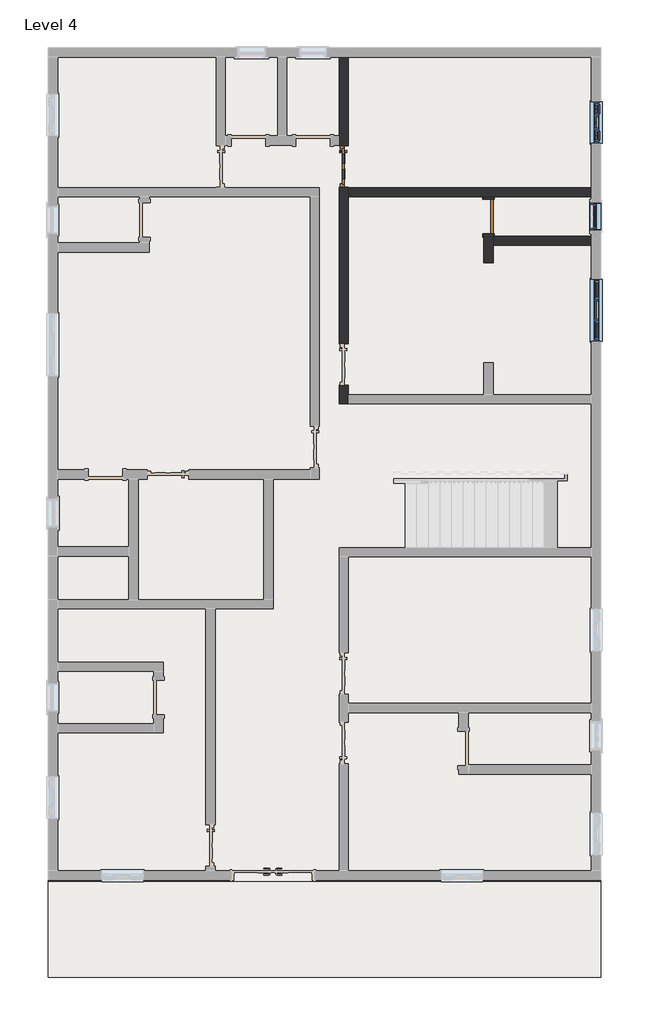
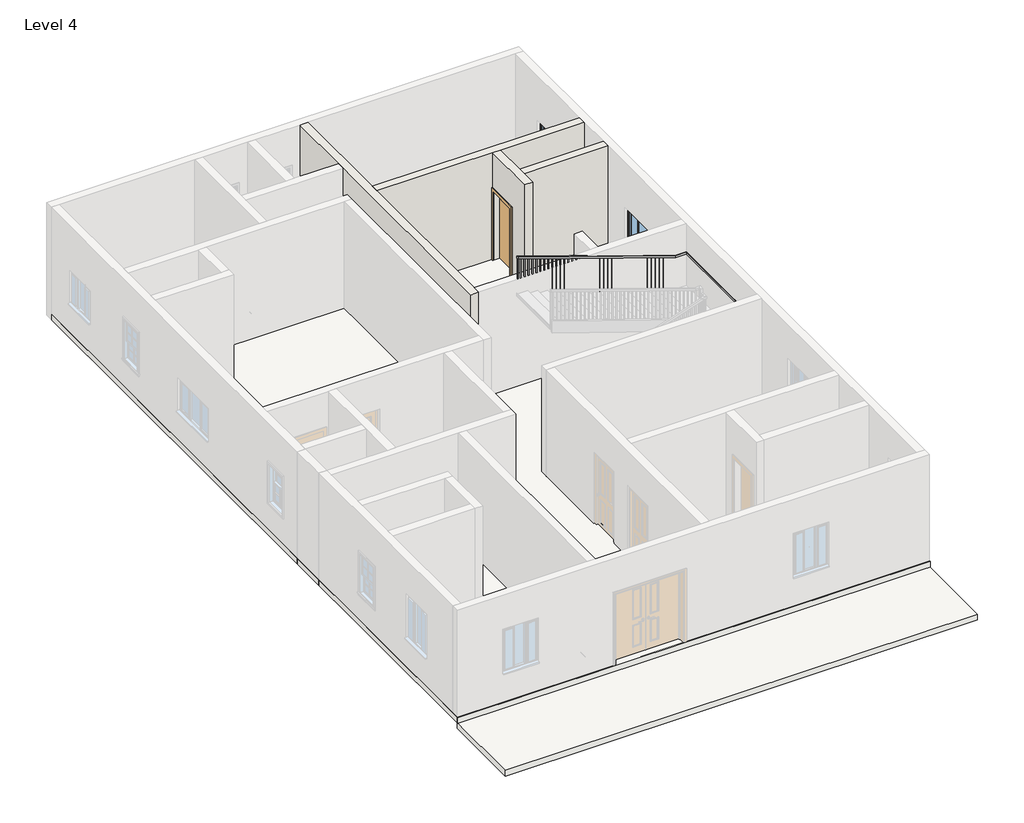
# One storey, part 2 of 3: 4 roofs, 4 walls, 3 windows, 2 doors, 1 railing, 1 slab.
"""IFC4 building model written with IfcOpenShell, lengths in millimetres."""

from ifc_helpers import new_model, si_unit, frame, origin, place, context, project, spatial, polyline, outline, extrude, faceted_brep, transform, mapped, element, save
from components import door_51b0c682, door_fadea3f2, window_679d2811, windows_tpl_plain_1360x910mm_84993ef1, windows_tpl_w_glazing_cross_bars_910x910mm_4aa0f884

model = new_model("IFC4")

# Units and contexts
model_context = context("Model", 3, world=origin())
ifc_project = project(units=[si_unit("LENGTHUNIT", "METRE", prefix="MILLI")], contexts=[model_context])

# Site, building, storey
site = spatial("IfcSite", under=ifc_project)
building = spatial("IfcBuilding", under=site)
storey = spatial("IfcBuildingStorey", under=building, Name="Level 4", Elevation=9144.0)

# Doors
placement = place(None, origin())
door_shape = door_51b0c682(model_context)
element("IfcDoor", 1, ObjectType="Doors_ExtSgl_2 : 2'x7\"", at=placement, inside=storey, context=model_context, shape_type="MappedRepresentation", body=[
    mapped(door_shape, transform((348.5548051, 6357.8803322, 9144.0), x_axis=(0.0, -1.0, 0.0), y_axis=(1.0, 0.0, 0.0), z_axis=(0.0, 0.0, 1.0))),
])
door_2_shape = door_fadea3f2(model_context)
element("IfcDoor", 2, ObjectType="Single-Flush : 30\" x 80\"", at=placement, inside=storey, context=model_context, shape_type="MappedRepresentation", body=[
    mapped(door_2_shape, transform((3523.5548051, 5259.3303322, 9144.0), x_axis=(0.0, -1.0, 0.0), y_axis=(1.0, 0.0, 0.0), z_axis=(0.0, 0.0, 1.0))),
])

# Railing
element("IfcRailing", 3, ObjectType="Handrail - Rectangular", at=placement, inside=storey, context=model_context, shape_type="SolidModel", body=[
    faceted_brep([(1449.3932247, -2014.4659014, 10144.125), (1449.3932247, -2014.4659014, 10090.4913852), (1449.3932247, -2065.2659014, 10090.4913852), (1449.3932247, -2065.2659014, 10144.125), (5246.6669505, -2014.4659014, 11430.0), (5255.0348019, -2014.4659014, 11379.2), (5255.0348019, -2065.2659014, 11379.2), (5246.6669505, -2065.2659014, 11430.0), (5771.4548051, -2014.4659014, 11430.0), (5771.4548051, -2014.4659014, 11379.2), (5822.2548051, -2065.2659014, 11379.2), (5822.2548051, -2065.2659014, 11430.0), (5771.4548051, 1135.1340986, 11430.0), (5771.4548051, 1135.1340986, 11379.2), (5822.2548051, 1185.9340986, 11379.2), (5822.2548051, 1185.9340986, 11430.0), (5499.8185322, 1135.1340986, 11430.0), (5491.4506807, 1135.1340986, 11379.2), (5491.4506807, 1185.9340986, 11379.2), (5499.8185322, 1185.9340986, 11430.0), (1449.3932247, 1135.1340986, 12801.6), (1449.3932247, 1185.9340986, 12801.6), (1449.3932247, 1185.9340986, 12747.9663852), (1449.3932247, 1135.1340986, 12747.9663852)], [[[0, 1, 2, 3]], [[1, 0, 4, 5]], [[2, 1, 5, 6]], [[3, 2, 6, 7]], [[0, 3, 7, 4]], [[5, 4, 8, 9]], [[6, 5, 9, 10]], [[7, 6, 10, 11]], [[4, 7, 11, 8]], [[9, 8, 12, 13]], [[10, 9, 13, 14]], [[11, 10, 14, 15]], [[8, 11, 15, 12]], [[13, 12, 16, 17]], [[14, 13, 17, 18]], [[15, 14, 18, 19]], [[12, 15, 19, 16]], [[20, 21, 22, 23]], [[17, 16, 20, 23]], [[18, 17, 23, 22]], [[19, 18, 22, 21]], [[16, 19, 21, 20]]]),
    extrude(outline(polyline([(12717.5618562, 1539.1798051), (12724.0127788, 1520.1298051), (11801.475, 1520.1298051), (11801.475, 1539.1798051), (12717.5618562, 1539.1798051)])), frame((0.0, 1151.0090986, 0.0), z_axis=(0.0, 1.0, 0.0), x_axis=(0.0, 0.0, 1.0)), (0.0, 0.0, 1.0), 19.05),
    extrude(outline(polyline([(12683.1569359, 1640.7798051), (12689.6078585, 1621.7298051), (11801.475, 1621.7298051), (11801.475, 1640.7798051), (12683.1569359, 1640.7798051)])), frame((0.0, 1151.0090986, 0.0), z_axis=(0.0, 1.0, 0.0), x_axis=(0.0, 0.0, 1.0)), (0.0, 0.0, 1.0), 19.05),
    extrude(outline(polyline([(12648.7520156, 1742.3798051), (12655.2029381, 1723.3298051), (11715.75, 1723.3298051), (11715.75, 1742.3798051), (12648.7520156, 1742.3798051)])), frame((0.0, 1151.0090986, 0.0), z_axis=(0.0, 1.0, 0.0), x_axis=(0.0, 0.0, 1.0)), (0.0, 0.0, 1.0), 19.05),
    extrude(outline(polyline([(12614.3470953, 1843.9798051), (12620.7980178, 1824.9298051), (11715.75, 1824.9298051), (11715.75, 1843.9798051), (12614.3470953, 1843.9798051)])), frame((0.0, 1151.0090986, 0.0), z_axis=(0.0, 1.0, 0.0), x_axis=(0.0, 0.0, 1.0)), (0.0, 0.0, 1.0), 19.05),
    extrude(outline(polyline([(12579.9421749, 1945.5798051), (12586.3930975, 1926.5298051), (11715.75, 1926.5298051), (11715.75, 1945.5798051), (12579.9421749, 1945.5798051)])), frame((0.0, 1151.0090986, 0.0), z_axis=(0.0, 1.0, 0.0), x_axis=(0.0, 0.0, 1.0)), (0.0, 0.0, 1.0), 19.05),
    extrude(outline(polyline([(12545.5372546, 2047.1798051), (12551.9881772, 2028.1298051), (11630.025, 2028.1298051), (11630.025, 2047.1798051), (12545.5372546, 2047.1798051)])), frame((0.0, 1151.0090986, 0.0), z_axis=(0.0, 1.0, 0.0), x_axis=(0.0, 0.0, 1.0)), (0.0, 0.0, 1.0), 19.05),
    extrude(outline(polyline([(12511.1323343, 2148.7798051), (12517.5832568, 2129.7298051), (11630.025, 2129.7298051), (11630.025, 2148.7798051), (12511.1323343, 2148.7798051)])), frame((0.0, 1151.0090986, 0.0), z_axis=(0.0, 1.0, 0.0), x_axis=(0.0, 0.0, 1.0)), (0.0, 0.0, 1.0), 19.05),
    extrude(outline(polyline([(12476.7274139, 2250.3798051), (12483.1783365, 2231.3298051), (11544.3, 2231.3298051), (11544.3, 2250.3798051), (12476.7274139, 2250.3798051)])), frame((0.0, 1151.0090986, 0.0), z_axis=(0.0, 1.0, 0.0), x_axis=(0.0, 0.0, 1.0)), (0.0, 0.0, 1.0), 19.05),
    extrude(outline(polyline([(12442.3224936, 2351.9798051), (12448.7734162, 2332.9298051), (11544.3, 2332.9298051), (11544.3, 2351.9798051), (12442.3224936, 2351.9798051)])), frame((0.0, 1151.0090986, 0.0), z_axis=(0.0, 1.0, 0.0), x_axis=(0.0, 0.0, 1.0)), (0.0, 0.0, 1.0), 19.05),
    extrude(outline(polyline([(12407.9175733, 2453.5798051), (12414.3684958, 2434.5298051), (11544.3, 2434.5298051), (11544.3, 2453.5798051), (12407.9175733, 2453.5798051)])), frame((0.0, 1151.0090986, 0.0), z_axis=(0.0, 1.0, 0.0), x_axis=(0.0, 0.0, 1.0)), (0.0, 0.0, 1.0), 19.05),
    extrude(outline(polyline([(12373.512653, 2555.1798051), (12379.9635755, 2536.1298051), (11458.575, 2536.1298051), (11458.575, 2555.1798051), (12373.512653, 2555.1798051)])), frame((0.0, 1151.0090986, 0.0), z_axis=(0.0, 1.0, 0.0), x_axis=(0.0, 0.0, 1.0)), (0.0, 0.0, 1.0), 19.05),
    extrude(outline(polyline([(12339.1077326, 2656.7798051), (12345.5586552, 2637.7298051), (11458.575, 2637.7298051), (11458.575, 2656.7798051), (12339.1077326, 2656.7798051)])), frame((0.0, 1151.0090986, 0.0), z_axis=(0.0, 1.0, 0.0), x_axis=(0.0, 0.0, 1.0)), (0.0, 0.0, 1.0), 19.05),
    extrude(outline(polyline([(12304.7028123, 2758.3798051), (12311.1537349, 2739.3298051), (11372.85, 2739.3298051), (11372.85, 2758.3798051), (12304.7028123, 2758.3798051)])), frame((0.0, 1151.0090986, 0.0), z_axis=(0.0, 1.0, 0.0), x_axis=(0.0, 0.0, 1.0)), (0.0, 0.0, 1.0), 19.05),
    extrude(outline(polyline([(12270.297892, 2859.9798051), (12276.7488145, 2840.9298051), (11372.85, 2840.9298051), (11372.85, 2859.9798051), (12270.297892, 2859.9798051)])), frame((0.0, 1151.0090986, 0.0), z_axis=(0.0, 1.0, 0.0), x_axis=(0.0, 0.0, 1.0)), (0.0, 0.0, 1.0), 19.05),
    extrude(outline(polyline([(12235.8929716, 2961.5798051), (12242.3438942, 2942.5298051), (11372.85, 2942.5298051), (11372.85, 2961.5798051), (12235.8929716, 2961.5798051)])), frame((0.0, 1151.0090986, 0.0), z_axis=(0.0, 1.0, 0.0), x_axis=(0.0, 0.0, 1.0)), (0.0, 0.0, 1.0), 19.05),
    extrude(outline(polyline([(12201.4880513, 3063.1798051), (12207.9389739, 3044.1298051), (11287.125, 3044.1298051), (11287.125, 3063.1798051), (12201.4880513, 3063.1798051)])), frame((0.0, 1151.0090986, 0.0), z_axis=(0.0, 1.0, 0.0), x_axis=(0.0, 0.0, 1.0)), (0.0, 0.0, 1.0), 19.05),
    extrude(outline(polyline([(12167.083131, 3164.7798051), (12173.5340535, 3145.7298051), (11287.125, 3145.7298051), (11287.125, 3164.7798051), (12167.083131, 3164.7798051)])), frame((0.0, 1151.0090986, 0.0), z_axis=(0.0, 1.0, 0.0), x_axis=(0.0, 0.0, 1.0)), (0.0, 0.0, 1.0), 19.05),
    extrude(outline(polyline([(12132.6782106, 3266.3798051), (12139.1291332, 3247.3298051), (11201.4, 3247.3298051), (11201.4, 3266.3798051), (12132.6782106, 3266.3798051)])), frame((0.0, 1151.0090986, 0.0), z_axis=(0.0, 1.0, 0.0), x_axis=(0.0, 0.0, 1.0)), (0.0, 0.0, 1.0), 19.05),
    extrude(outline(polyline([(12098.2732903, 3367.9798051), (12104.7242129, 3348.9298051), (11201.4, 3348.9298051), (11201.4, 3367.9798051), (12098.2732903, 3367.9798051)])), frame((0.0, 1151.0090986, 0.0), z_axis=(0.0, 1.0, 0.0), x_axis=(0.0, 0.0, 1.0)), (0.0, 0.0, 1.0), 19.05),
    extrude(outline(polyline([(12063.86837, 3469.5798051), (12070.3192926, 3450.5298051), (11201.4, 3450.5298051), (11201.4, 3469.5798051), (12063.86837, 3469.5798051)])), frame((0.0, 1151.0090986, 0.0), z_axis=(0.0, 1.0, 0.0), x_axis=(0.0, 0.0, 1.0)), (0.0, 0.0, 1.0), 19.05),
    extrude(outline(polyline([(12029.4634497, 3571.1798051), (12035.9143722, 3552.1298051), (11115.675, 3552.1298051), (11115.675, 3571.1798051), (12029.4634497, 3571.1798051)])), frame((0.0, 1151.0090986, 0.0), z_axis=(0.0, 1.0, 0.0), x_axis=(0.0, 0.0, 1.0)), (0.0, 0.0, 1.0), 19.05),
    extrude(outline(polyline([(11995.0585293, 3672.7798051), (12001.5094519, 3653.7298051), (11115.675, 3653.7298051), (11115.675, 3672.7798051), (11995.0585293, 3672.7798051)])), frame((0.0, 1151.0090986, 0.0), z_axis=(0.0, 1.0, 0.0), x_axis=(0.0, 0.0, 1.0)), (0.0, 0.0, 1.0), 19.05),
    extrude(outline(polyline([(11960.653609, 3774.3798051), (11967.1045316, 3755.3298051), (11029.95, 3755.3298051), (11029.95, 3774.3798051), (11960.653609, 3774.3798051)])), frame((0.0, 1151.0090986, 0.0), z_axis=(0.0, 1.0, 0.0), x_axis=(0.0, 0.0, 1.0)), (0.0, 0.0, 1.0), 19.05),
    extrude(outline(polyline([(11926.2486887, 3875.9798051), (11932.6996112, 3856.9298051), (11029.95, 3856.9298051), (11029.95, 3875.9798051), (11926.2486887, 3875.9798051)])), frame((0.0, 1151.0090986, 0.0), z_axis=(0.0, 1.0, 0.0), x_axis=(0.0, 0.0, 1.0)), (0.0, 0.0, 1.0), 19.05),
    extrude(outline(polyline([(11891.8437683, 3977.5798051), (11898.2946909, 3958.5298051), (11029.95, 3958.5298051), (11029.95, 3977.5798051), (11891.8437683, 3977.5798051)])), frame((0.0, 1151.0090986, 0.0), z_axis=(0.0, 1.0, 0.0), x_axis=(0.0, 0.0, 1.0)), (0.0, 0.0, 1.0), 19.05),
    extrude(outline(polyline([(11857.438848, 4079.1798051), (11863.8897706, 4060.1298051), (10944.225, 4060.1298051), (10944.225, 4079.1798051), (11857.438848, 4079.1798051)])), frame((0.0, 1151.0090986, 0.0), z_axis=(0.0, 1.0, 0.0), x_axis=(0.0, 0.0, 1.0)), (0.0, 0.0, 1.0), 19.05),
    extrude(outline(polyline([(11823.0339277, 4180.7798051), (11829.4848502, 4161.7298051), (10944.225, 4161.7298051), (10944.225, 4180.7798051), (11823.0339277, 4180.7798051)])), frame((0.0, 1151.0090986, 0.0), z_axis=(0.0, 1.0, 0.0), x_axis=(0.0, 0.0, 1.0)), (0.0, 0.0, 1.0), 19.05),
    extrude(outline(polyline([(11788.6290074, 4282.3798051), (11795.0799299, 4263.3298051), (10858.5, 4263.3298051), (10858.5, 4282.3798051), (11788.6290074, 4282.3798051)])), frame((0.0, 1151.0090986, 0.0), z_axis=(0.0, 1.0, 0.0), x_axis=(0.0, 0.0, 1.0)), (0.0, 0.0, 1.0), 19.05),
    extrude(outline(polyline([(11754.224087, 4383.9798051), (11760.6750096, 4364.9298051), (10858.5, 4364.9298051), (10858.5, 4383.9798051), (11754.224087, 4383.9798051)])), frame((0.0, 1151.0090986, 0.0), z_axis=(0.0, 1.0, 0.0), x_axis=(0.0, 0.0, 1.0)), (0.0, 0.0, 1.0), 19.05),
    extrude(outline(polyline([(11719.8191667, 4485.5798051), (11726.2700893, 4466.5298051), (10858.5, 4466.5298051), (10858.5, 4485.5798051), (11719.8191667, 4485.5798051)])), frame((0.0, 1151.0090986, 0.0), z_axis=(0.0, 1.0, 0.0), x_axis=(0.0, 0.0, 1.0)), (0.0, 0.0, 1.0), 19.05),
    extrude(outline(polyline([(11685.4142464, 4587.1798051), (11691.8651689, 4568.1298051), (10772.775, 4568.1298051), (10772.775, 4587.1798051), (11685.4142464, 4587.1798051)])), frame((0.0, 1151.0090986, 0.0), z_axis=(0.0, 1.0, 0.0), x_axis=(0.0, 0.0, 1.0)), (0.0, 0.0, 1.0), 19.05),
    extrude(outline(polyline([(11651.009326, 4688.7798051), (11657.4602486, 4669.7298051), (10772.775, 4669.7298051), (10772.775, 4688.7798051), (11651.009326, 4688.7798051)])), frame((0.0, 1151.0090986, 0.0), z_axis=(0.0, 1.0, 0.0), x_axis=(0.0, 0.0, 1.0)), (0.0, 0.0, 1.0), 19.05),
    extrude(outline(polyline([(11616.6044057, 4790.3798051), (11623.0553283, 4771.3298051), (10687.05, 4771.3298051), (10687.05, 4790.3798051), (11616.6044057, 4790.3798051)])), frame((0.0, 1151.0090986, 0.0), z_axis=(0.0, 1.0, 0.0), x_axis=(0.0, 0.0, 1.0)), (0.0, 0.0, 1.0), 19.05),
    extrude(outline(polyline([(11582.1994854, 4891.9798051), (11588.6504079, 4872.9298051), (10687.05, 4872.9298051), (10687.05, 4891.9798051), (11582.1994854, 4891.9798051)])), frame((0.0, 1151.0090986, 0.0), z_axis=(0.0, 1.0, 0.0), x_axis=(0.0, 0.0, 1.0)), (0.0, 0.0, 1.0), 19.05),
    extrude(outline(polyline([(11547.8163852, 4993.5798051), (11554.2673078, 4974.5298051), (10687.05, 4974.5298051), (10687.05, 4993.5798051), (11547.8163852, 4993.5798051)])), frame((0.0, 1151.0090986, 0.0), z_axis=(0.0, 1.0, 0.0), x_axis=(0.0, 0.0, 1.0)), (0.0, 0.0, 1.0), 19.05),
    extrude(outline(polyline([(11513.3896447, 5095.1798051), (11519.8405673, 5076.1298051), (10601.325, 5076.1298051), (10601.325, 5095.1798051), (11513.3896447, 5095.1798051)])), frame((0.0, 1151.0090986, 0.0), z_axis=(0.0, 1.0, 0.0), x_axis=(0.0, 0.0, 1.0)), (0.0, 0.0, 1.0), 19.05),
    extrude(outline(polyline([(11478.9847244, 5196.7798051), (11485.435647, 5177.7298051), (10601.325, 5177.7298051), (10601.325, 5196.7798051), (11478.9847244, 5196.7798051)])), frame((0.0, 1151.0090986, 0.0), z_axis=(0.0, 1.0, 0.0), x_axis=(0.0, 0.0, 1.0)), (0.0, 0.0, 1.0), 19.05),
    extrude(outline(polyline([(11444.5798041, 5298.3798051), (11451.0307266, 5279.3298051), (10515.6, 5279.3298051), (10515.6, 5298.3798051), (11444.5798041, 5298.3798051)])), frame((0.0, 1151.0090986, 0.0), z_axis=(0.0, 1.0, 0.0), x_axis=(0.0, 0.0, 1.0)), (0.0, 0.0, 1.0), 19.05),
    extrude(outline(polyline([(11410.1748837, 5399.9798051), (11416.6258063, 5380.9298051), (10515.6, 5380.9298051), (10515.6, 5399.9798051), (11410.1748837, 5399.9798051)])), frame((0.0, 1151.0090986, 0.0), z_axis=(0.0, 1.0, 0.0), x_axis=(0.0, 0.0, 1.0)), (0.0, 0.0, 1.0), 19.05),
    extrude(outline(polyline([(11375.7699634, 5501.5798051), (11382.220886, 5482.5298051), (10515.6, 5482.5298051), (10515.6, 5501.5798051), (11375.7699634, 5501.5798051)])), frame((0.0, 1151.0090986, 0.0), z_axis=(0.0, 1.0, 0.0), x_axis=(0.0, 0.0, 1.0)), (0.0, 0.0, 1.0), 19.05),
    extrude(outline(polyline([(5603.1798051, 1170.0590986), (5603.1798051, 1151.0090986), (5584.1298051, 1151.0090986), (5584.1298051, 1170.0590986), (5603.1798051, 1170.0590986)])), frame((0.0, 0.0, 10515.6), z_axis=(0.0, 0.0, 1.0), x_axis=(1.0, 0.0, 0.0)), (0.0, 0.0, 1.0), 863.6),
    extrude(outline(polyline([(5704.7798051, 1170.0590986), (5704.7798051, 1151.0090986), (5685.7298051, 1151.0090986), (5685.7298051, 1170.0590986), (5704.7798051, 1170.0590986)])), frame((0.0, 0.0, 10515.6), z_axis=(0.0, 0.0, 1.0), x_axis=(1.0, 0.0, 0.0)), (0.0, 0.0, 1.0), 863.6),
    extrude(outline(polyline([(5806.3798051, 1100.2090986), (5787.3298051, 1100.2090986), (5787.3298051, 1119.2590986), (5806.3798051, 1119.2590986), (5806.3798051, 1100.2090986)])), frame((0.0, 0.0, 10515.6), z_axis=(0.0, 0.0, 1.0), x_axis=(1.0, 0.0, 0.0)), (0.0, 0.0, 1.0), 863.6),
    extrude(outline(polyline([(5806.3798051, 998.6090986), (5787.3298051, 998.6090986), (5787.3298051, 1017.6590986), (5806.3798051, 1017.6590986), (5806.3798051, 998.6090986)])), frame((0.0, 0.0, 10515.6), z_axis=(0.0, 0.0, 1.0), x_axis=(1.0, 0.0, 0.0)), (0.0, 0.0, 1.0), 863.6),
    extrude(outline(polyline([(5806.3798051, 897.0090986), (5787.3298051, 897.0090986), (5787.3298051, 916.0590986), (5806.3798051, 916.0590986), (5806.3798051, 897.0090986)])), frame((0.0, 0.0, 10515.6), z_axis=(0.0, 0.0, 1.0), x_axis=(1.0, 0.0, 0.0)), (0.0, 0.0, 1.0), 863.6),
    extrude(outline(polyline([(5806.3798051, 795.4090986), (5787.3298051, 795.4090986), (5787.3298051, 814.4590986), (5806.3798051, 814.4590986), (5806.3798051, 795.4090986)])), frame((0.0, 0.0, 10515.6), z_axis=(0.0, 0.0, 1.0), x_axis=(1.0, 0.0, 0.0)), (0.0, 0.0, 1.0), 863.6),
    extrude(outline(polyline([(5806.3798051, 693.8090986), (5787.3298051, 693.8090986), (5787.3298051, 712.8590986), (5806.3798051, 712.8590986), (5806.3798051, 693.8090986)])), frame((0.0, 0.0, 10515.6), z_axis=(0.0, 0.0, 1.0), x_axis=(1.0, 0.0, 0.0)), (0.0, 0.0, 1.0), 863.6),
    extrude(outline(polyline([(5806.3798051, 592.2090986), (5787.3298051, 592.2090986), (5787.3298051, 611.2590986), (5806.3798051, 611.2590986), (5806.3798051, 592.2090986)])), frame((0.0, 0.0, 10515.6), z_axis=(0.0, 0.0, 1.0), x_axis=(1.0, 0.0, 0.0)), (0.0, 0.0, 1.0), 863.6),
    extrude(outline(polyline([(5806.3798051, 490.6090986), (5787.3298051, 490.6090986), (5787.3298051, 509.6590986), (5806.3798051, 509.6590986), (5806.3798051, 490.6090986)])), frame((0.0, 0.0, 10515.6), z_axis=(0.0, 0.0, 1.0), x_axis=(1.0, 0.0, 0.0)), (0.0, 0.0, 1.0), 863.6),
    extrude(outline(polyline([(5806.3798051, 389.0090986), (5787.3298051, 389.0090986), (5787.3298051, 408.0590986), (5806.3798051, 408.0590986), (5806.3798051, 389.0090986)])), frame((0.0, 0.0, 10515.6), z_axis=(0.0, 0.0, 1.0), x_axis=(1.0, 0.0, 0.0)), (0.0, 0.0, 1.0), 863.6),
    extrude(outline(polyline([(5806.3798051, 287.4090986), (5787.3298051, 287.4090986), (5787.3298051, 306.4590986), (5806.3798051, 306.4590986), (5806.3798051, 287.4090986)])), frame((0.0, 0.0, 10515.6), z_axis=(0.0, 0.0, 1.0), x_axis=(1.0, 0.0, 0.0)), (0.0, 0.0, 1.0), 863.6),
    extrude(outline(polyline([(5806.3798051, 185.8090986), (5787.3298051, 185.8090986), (5787.3298051, 204.8590986), (5806.3798051, 204.8590986), (5806.3798051, 185.8090986)])), frame((0.0, 0.0, 10515.6), z_axis=(0.0, 0.0, 1.0), x_axis=(1.0, 0.0, 0.0)), (0.0, 0.0, 1.0), 863.6),
    extrude(outline(polyline([(5806.3798051, 84.2090986), (5787.3298051, 84.2090986), (5787.3298051, 103.2590986), (5806.3798051, 103.2590986), (5806.3798051, 84.2090986)])), frame((0.0, 0.0, 10515.6), z_axis=(0.0, 0.0, 1.0), x_axis=(1.0, 0.0, 0.0)), (0.0, 0.0, 1.0), 863.6),
    extrude(outline(polyline([(5806.3798051, -17.3909014), (5787.3298051, -17.3909014), (5787.3298051, 1.6590986), (5806.3798051, 1.6590986), (5806.3798051, -17.3909014)])), frame((0.0, 0.0, 10515.6), z_axis=(0.0, 0.0, 1.0), x_axis=(1.0, 0.0, 0.0)), (0.0, 0.0, 1.0), 863.6),
    extrude(outline(polyline([(5806.3798051, -118.9909014), (5787.3298051, -118.9909014), (5787.3298051, -99.9409014), (5806.3798051, -99.9409014), (5806.3798051, -118.9909014)])), frame((0.0, 0.0, 10515.6), z_axis=(0.0, 0.0, 1.0), x_axis=(1.0, 0.0, 0.0)), (0.0, 0.0, 1.0), 863.6),
    extrude(outline(polyline([(5806.3798051, -220.5909014), (5787.3298051, -220.5909014), (5787.3298051, -201.5409014), (5806.3798051, -201.5409014), (5806.3798051, -220.5909014)])), frame((0.0, 0.0, 10515.6), z_axis=(0.0, 0.0, 1.0), x_axis=(1.0, 0.0, 0.0)), (0.0, 0.0, 1.0), 863.6),
    extrude(outline(polyline([(5806.3798051, -322.1909014), (5787.3298051, -322.1909014), (5787.3298051, -303.1409014), (5806.3798051, -303.1409014), (5806.3798051, -322.1909014)])), frame((0.0, 0.0, 10515.6), z_axis=(0.0, 0.0, 1.0), x_axis=(1.0, 0.0, 0.0)), (0.0, 0.0, 1.0), 863.6),
    extrude(outline(polyline([(5806.3798051, -423.7909014), (5787.3298051, -423.7909014), (5787.3298051, -404.7409014), (5806.3798051, -404.7409014), (5806.3798051, -423.7909014)])), frame((0.0, 0.0, 10515.6), z_axis=(0.0, 0.0, 1.0), x_axis=(1.0, 0.0, 0.0)), (0.0, 0.0, 1.0), 863.6),
    extrude(outline(polyline([(5806.3798051, -525.3909014), (5787.3298051, -525.3909014), (5787.3298051, -506.3409014), (5806.3798051, -506.3409014), (5806.3798051, -525.3909014)])), frame((0.0, 0.0, 10515.6), z_axis=(0.0, 0.0, 1.0), x_axis=(1.0, 0.0, 0.0)), (0.0, 0.0, 1.0), 863.6),
    extrude(outline(polyline([(5806.3798051, -626.9909014), (5787.3298051, -626.9909014), (5787.3298051, -607.9409014), (5806.3798051, -607.9409014), (5806.3798051, -626.9909014)])), frame((0.0, 0.0, 10515.6), z_axis=(0.0, 0.0, 1.0), x_axis=(1.0, 0.0, 0.0)), (0.0, 0.0, 1.0), 863.6),
    extrude(outline(polyline([(5806.3798051, -728.5909014), (5787.3298051, -728.5909014), (5787.3298051, -709.5409014), (5806.3798051, -709.5409014), (5806.3798051, -728.5909014)])), frame((0.0, 0.0, 10515.6), z_axis=(0.0, 0.0, 1.0), x_axis=(1.0, 0.0, 0.0)), (0.0, 0.0, 1.0), 863.6),
    extrude(outline(polyline([(5806.3798051, -830.1909014), (5787.3298051, -830.1909014), (5787.3298051, -811.1409014), (5806.3798051, -811.1409014), (5806.3798051, -830.1909014)])), frame((0.0, 0.0, 10515.6), z_axis=(0.0, 0.0, 1.0), x_axis=(1.0, 0.0, 0.0)), (0.0, 0.0, 1.0), 863.6),
    extrude(outline(polyline([(5806.3798051, -931.7909014), (5787.3298051, -931.7909014), (5787.3298051, -912.7409014), (5806.3798051, -912.7409014), (5806.3798051, -931.7909014)])), frame((0.0, 0.0, 10515.6), z_axis=(0.0, 0.0, 1.0), x_axis=(1.0, 0.0, 0.0)), (0.0, 0.0, 1.0), 863.6),
    extrude(outline(polyline([(5806.3798051, -1033.3909014), (5787.3298051, -1033.3909014), (5787.3298051, -1014.3409014), (5806.3798051, -1014.3409014), (5806.3798051, -1033.3909014)])), frame((0.0, 0.0, 10515.6), z_axis=(0.0, 0.0, 1.0), x_axis=(1.0, 0.0, 0.0)), (0.0, 0.0, 1.0), 863.6),
    extrude(outline(polyline([(5806.3798051, -1134.9909014), (5787.3298051, -1134.9909014), (5787.3298051, -1115.9409014), (5806.3798051, -1115.9409014), (5806.3798051, -1134.9909014)])), frame((0.0, 0.0, 10515.6), z_axis=(0.0, 0.0, 1.0), x_axis=(1.0, 0.0, 0.0)), (0.0, 0.0, 1.0), 863.6),
    extrude(outline(polyline([(5806.3798051, -1236.5909014), (5787.3298051, -1236.5909014), (5787.3298051, -1217.5409014), (5806.3798051, -1217.5409014), (5806.3798051, -1236.5909014)])), frame((0.0, 0.0, 10515.6), z_axis=(0.0, 0.0, 1.0), x_axis=(1.0, 0.0, 0.0)), (0.0, 0.0, 1.0), 863.6),
    extrude(outline(polyline([(5806.3798051, -1338.1909014), (5787.3298051, -1338.1909014), (5787.3298051, -1319.1409014), (5806.3798051, -1319.1409014), (5806.3798051, -1338.1909014)])), frame((0.0, 0.0, 10515.6), z_axis=(0.0, 0.0, 1.0), x_axis=(1.0, 0.0, 0.0)), (0.0, 0.0, 1.0), 863.6),
    extrude(outline(polyline([(5806.3798051, -1439.7909014), (5787.3298051, -1439.7909014), (5787.3298051, -1420.7409014), (5806.3798051, -1420.7409014), (5806.3798051, -1439.7909014)])), frame((0.0, 0.0, 10515.6), z_axis=(0.0, 0.0, 1.0), x_axis=(1.0, 0.0, 0.0)), (0.0, 0.0, 1.0), 863.6),
    extrude(outline(polyline([(5806.3798051, -1541.3909014), (5787.3298051, -1541.3909014), (5787.3298051, -1522.3409014), (5806.3798051, -1522.3409014), (5806.3798051, -1541.3909014)])), frame((0.0, 0.0, 10515.6), z_axis=(0.0, 0.0, 1.0), x_axis=(1.0, 0.0, 0.0)), (0.0, 0.0, 1.0), 863.6),
    extrude(outline(polyline([(5806.3798051, -1642.9909014), (5787.3298051, -1642.9909014), (5787.3298051, -1623.9409014), (5806.3798051, -1623.9409014), (5806.3798051, -1642.9909014)])), frame((0.0, 0.0, 10515.6), z_axis=(0.0, 0.0, 1.0), x_axis=(1.0, 0.0, 0.0)), (0.0, 0.0, 1.0), 863.6),
    extrude(outline(polyline([(5806.3798051, -1744.5909014), (5787.3298051, -1744.5909014), (5787.3298051, -1725.5409014), (5806.3798051, -1725.5409014), (5806.3798051, -1744.5909014)])), frame((0.0, 0.0, 10515.6), z_axis=(0.0, 0.0, 1.0), x_axis=(1.0, 0.0, 0.0)), (0.0, 0.0, 1.0), 863.6),
    extrude(outline(polyline([(5806.3798051, -1846.1909014), (5787.3298051, -1846.1909014), (5787.3298051, -1827.1409014), (5806.3798051, -1827.1409014), (5806.3798051, -1846.1909014)])), frame((0.0, 0.0, 10515.6), z_axis=(0.0, 0.0, 1.0), x_axis=(1.0, 0.0, 0.0)), (0.0, 0.0, 1.0), 863.6),
    extrude(outline(polyline([(5806.3798051, -1947.7909014), (5787.3298051, -1947.7909014), (5787.3298051, -1928.7409014), (5806.3798051, -1928.7409014), (5806.3798051, -1947.7909014)])), frame((0.0, 0.0, 10515.6), z_axis=(0.0, 0.0, 1.0), x_axis=(1.0, 0.0, 0.0)), (0.0, 0.0, 1.0), 863.6),
    extrude(outline(polyline([(5707.0682247, -2049.3909014), (5707.0682247, -2030.3409014), (5726.1182247, -2030.3409014), (5726.1182247, -2049.3909014), (5707.0682247, -2049.3909014)])), frame((0.0, 0.0, 10515.6), z_axis=(0.0, 0.0, 1.0), x_axis=(1.0, 0.0, 0.0)), (0.0, 0.0, 1.0), 863.6),
    extrude(outline(polyline([(5605.4682247, -2049.3909014), (5605.4682247, -2030.3409014), (5624.5182247, -2030.3409014), (5624.5182247, -2049.3909014), (5605.4682247, -2049.3909014)])), frame((0.0, 0.0, 10515.6), z_axis=(0.0, 0.0, 1.0), x_axis=(1.0, 0.0, 0.0)), (0.0, 0.0, 1.0), 863.6),
    extrude(outline(polyline([(5503.8682247, -2049.3909014), (5503.8682247, -2030.3409014), (5522.9182247, -2030.3409014), (5522.9182247, -2049.3909014), (5503.8682247, -2049.3909014)])), frame((0.0, 0.0, 10515.6), z_axis=(0.0, 0.0, 1.0), x_axis=(1.0, 0.0, 0.0)), (0.0, 0.0, 1.0), 863.6),
    extrude(outline(polyline([(5402.2682247, -2049.3909014), (5402.2682247, -2030.3409014), (5421.3182247, -2030.3409014), (5421.3182247, -2049.3909014), (5402.2682247, -2049.3909014)])), frame((0.0, 0.0, 10515.6), z_axis=(0.0, 0.0, 1.0), x_axis=(1.0, 0.0, 0.0)), (0.0, 0.0, 1.0), 863.6),
    extrude(outline(polyline([(5300.6682247, -2049.3909014), (5300.6682247, -2030.3409014), (5319.7182247, -2030.3409014), (5319.7182247, -2049.3909014), (5300.6682247, -2049.3909014)])), frame((0.0, 0.0, 10515.6), z_axis=(0.0, 0.0, 1.0), x_axis=(1.0, 0.0, 0.0)), (0.0, 0.0, 1.0), 863.6),
    extrude(outline(polyline([(11366.6988987, 5218.1182247), (11360.2479761, 5199.0682247), (10429.875, 5199.0682247), (10429.875, 5218.1182247), (11366.6988987, 5218.1182247)])), frame((0.0, -2049.3909014, 0.0), z_axis=(0.0, 1.0, 0.0), x_axis=(0.0, 0.0, 1.0)), (0.0, 0.0, 1.0), 19.05),
    extrude(outline(polyline([(11332.2939783, 5116.5182247), (11325.8430558, 5097.4682247), (10429.875, 5097.4682247), (10429.875, 5116.5182247), (11332.2939783, 5116.5182247)])), frame((0.0, -2049.3909014, 0.0), z_axis=(0.0, 1.0, 0.0), x_axis=(0.0, 0.0, 1.0)), (0.0, 0.0, 1.0), 19.05),
    extrude(outline(polyline([(11297.889058, 5014.9182247), (11291.4381354, 4995.8682247), (10429.875, 4995.8682247), (10429.875, 5014.9182247), (11297.889058, 5014.9182247)])), frame((0.0, -2049.3909014, 0.0), z_axis=(0.0, 1.0, 0.0), x_axis=(0.0, 0.0, 1.0)), (0.0, 0.0, 1.0), 19.05),
    extrude(outline(polyline([(11263.4841377, 4913.3182247), (11257.0332151, 4894.2682247), (10344.15, 4894.2682247), (10344.15, 4913.3182247), (11263.4841377, 4913.3182247)])), frame((0.0, -2049.3909014, 0.0), z_axis=(0.0, 1.0, 0.0), x_axis=(0.0, 0.0, 1.0)), (0.0, 0.0, 1.0), 19.05),
    extrude(outline(polyline([(11229.0792173, 4811.7182247), (11222.6282948, 4792.6682247), (10344.15, 4792.6682247), (10344.15, 4811.7182247), (11229.0792173, 4811.7182247)])), frame((0.0, -2049.3909014, 0.0), z_axis=(0.0, 1.0, 0.0), x_axis=(0.0, 0.0, 1.0)), (0.0, 0.0, 1.0), 19.05),
    extrude(outline(polyline([(11194.674297, 4710.1182247), (11188.2233745, 4691.0682247), (10258.425, 4691.0682247), (10258.425, 4710.1182247), (11194.674297, 4710.1182247)])), frame((0.0, -2049.3909014, 0.0), z_axis=(0.0, 1.0, 0.0), x_axis=(0.0, 0.0, 1.0)), (0.0, 0.0, 1.0), 19.05),
    extrude(outline(polyline([(11160.2693767, 4608.5182247), (11153.8184541, 4589.4682247), (10258.425, 4589.4682247), (10258.425, 4608.5182247), (11160.2693767, 4608.5182247)])), frame((0.0, -2049.3909014, 0.0), z_axis=(0.0, 1.0, 0.0), x_axis=(0.0, 0.0, 1.0)), (0.0, 0.0, 1.0), 19.05),
    extrude(outline(polyline([(11125.8644564, 4506.9182247), (11119.4135338, 4487.8682247), (10258.425, 4487.8682247), (10258.425, 4506.9182247), (11125.8644564, 4506.9182247)])), frame((0.0, -2049.3909014, 0.0), z_axis=(0.0, 1.0, 0.0), x_axis=(0.0, 0.0, 1.0)), (0.0, 0.0, 1.0), 19.05),
    extrude(outline(polyline([(11091.459536, 4405.3182247), (11085.0086135, 4386.2682247), (10172.7, 4386.2682247), (10172.7, 4405.3182247), (11091.459536, 4405.3182247)])), frame((0.0, -2049.3909014, 0.0), z_axis=(0.0, 1.0, 0.0), x_axis=(0.0, 0.0, 1.0)), (0.0, 0.0, 1.0), 19.05),
    extrude(outline(polyline([(11057.0546157, 4303.7182247), (11050.6036931, 4284.6682247), (10172.7, 4284.6682247), (10172.7, 4303.7182247), (11057.0546157, 4303.7182247)])), frame((0.0, -2049.3909014, 0.0), z_axis=(0.0, 1.0, 0.0), x_axis=(0.0, 0.0, 1.0)), (0.0, 0.0, 1.0), 19.05),
    extrude(outline(polyline([(11022.6496954, 4202.1182247), (11016.1987728, 4183.0682247), (10086.975, 4183.0682247), (10086.975, 4202.1182247), (11022.6496954, 4202.1182247)])), frame((0.0, -2049.3909014, 0.0), z_axis=(0.0, 1.0, 0.0), x_axis=(0.0, 0.0, 1.0)), (0.0, 0.0, 1.0), 19.05),
    extrude(outline(polyline([(10988.244775, 4100.5182247), (10981.7938525, 4081.4682247), (10086.975, 4081.4682247), (10086.975, 4100.5182247), (10988.244775, 4100.5182247)])), frame((0.0, -2049.3909014, 0.0), z_axis=(0.0, 1.0, 0.0), x_axis=(0.0, 0.0, 1.0)), (0.0, 0.0, 1.0), 19.05),
    extrude(outline(polyline([(10953.8398547, 3998.9182247), (10947.3889321, 3979.8682247), (10086.975, 3979.8682247), (10086.975, 3998.9182247), (10953.8398547, 3998.9182247)])), frame((0.0, -2049.3909014, 0.0), z_axis=(0.0, 1.0, 0.0), x_axis=(0.0, 0.0, 1.0)), (0.0, 0.0, 1.0), 19.05),
    extrude(outline(polyline([(10919.4349344, 3897.3182247), (10912.9840118, 3878.2682247), (10001.25, 3878.2682247), (10001.25, 3897.3182247), (10919.4349344, 3897.3182247)])), frame((0.0, -2049.3909014, 0.0), z_axis=(0.0, 1.0, 0.0), x_axis=(0.0, 0.0, 1.0)), (0.0, 0.0, 1.0), 19.05),
    extrude(outline(polyline([(10885.0300141, 3795.7182247), (10878.5790915, 3776.6682247), (10001.25, 3776.6682247), (10001.25, 3795.7182247), (10885.0300141, 3795.7182247)])), frame((0.0, -2049.3909014, 0.0), z_axis=(0.0, 1.0, 0.0), x_axis=(0.0, 0.0, 1.0)), (0.0, 0.0, 1.0), 19.05),
    extrude(outline(polyline([(10850.6250937, 3694.1182247), (10844.1741712, 3675.0682247), (9915.525, 3675.0682247), (9915.525, 3694.1182247), (10850.6250937, 3694.1182247)])), frame((0.0, -2049.3909014, 0.0), z_axis=(0.0, 1.0, 0.0), x_axis=(0.0, 0.0, 1.0)), (0.0, 0.0, 1.0), 19.05),
    extrude(outline(polyline([(10816.2201734, 3592.5182247), (10809.7692508, 3573.4682247), (9915.525, 3573.4682247), (9915.525, 3592.5182247), (10816.2201734, 3592.5182247)])), frame((0.0, -2049.3909014, 0.0), z_axis=(0.0, 1.0, 0.0), x_axis=(0.0, 0.0, 1.0)), (0.0, 0.0, 1.0), 19.05),
    extrude(outline(polyline([(10781.8152531, 3490.9182247), (10775.3643305, 3471.8682247), (9915.525, 3471.8682247), (9915.525, 3490.9182247), (10781.8152531, 3490.9182247)])), frame((0.0, -2049.3909014, 0.0), z_axis=(0.0, 1.0, 0.0), x_axis=(0.0, 0.0, 1.0)), (0.0, 0.0, 1.0), 19.05),
    extrude(outline(polyline([(10747.4103327, 3389.3182247), (10740.9594102, 3370.2682247), (9829.8, 3370.2682247), (9829.8, 3389.3182247), (10747.4103327, 3389.3182247)])), frame((0.0, -2049.3909014, 0.0), z_axis=(0.0, 1.0, 0.0), x_axis=(0.0, 0.0, 1.0)), (0.0, 0.0, 1.0), 19.05),
    extrude(outline(polyline([(10713.0054124, 3287.7182247), (10706.5544898, 3268.6682247), (9829.8, 3268.6682247), (9829.8, 3287.7182247), (10713.0054124, 3287.7182247)])), frame((0.0, -2049.3909014, 0.0), z_axis=(0.0, 1.0, 0.0), x_axis=(0.0, 0.0, 1.0)), (0.0, 0.0, 1.0), 19.05),
    extrude(outline(polyline([(10678.6004921, 3186.1182247), (10672.1495695, 3167.0682247), (9744.075, 3167.0682247), (9744.075, 3186.1182247), (10678.6004921, 3186.1182247)])), frame((0.0, -2049.3909014, 0.0), z_axis=(0.0, 1.0, 0.0), x_axis=(0.0, 0.0, 1.0)), (0.0, 0.0, 1.0), 19.05),
    extrude(outline(polyline([(10644.1955718, 3084.5182247), (10637.7446492, 3065.4682247), (9744.075, 3065.4682247), (9744.075, 3084.5182247), (10644.1955718, 3084.5182247)])), frame((0.0, -2049.3909014, 0.0), z_axis=(0.0, 1.0, 0.0), x_axis=(0.0, 0.0, 1.0)), (0.0, 0.0, 1.0), 19.05),
    extrude(outline(polyline([(10609.7906514, 2982.9182247), (10603.3397289, 2963.8682247), (9744.075, 2963.8682247), (9744.075, 2982.9182247), (10609.7906514, 2982.9182247)])), frame((0.0, -2049.3909014, 0.0), z_axis=(0.0, 1.0, 0.0), x_axis=(0.0, 0.0, 1.0)), (0.0, 0.0, 1.0), 19.05),
    extrude(outline(polyline([(10575.3857311, 2881.3182247), (10568.9348085, 2862.2682247), (9658.35, 2862.2682247), (9658.35, 2881.3182247), (10575.3857311, 2881.3182247)])), frame((0.0, -2049.3909014, 0.0), z_axis=(0.0, 1.0, 0.0), x_axis=(0.0, 0.0, 1.0)), (0.0, 0.0, 1.0), 19.05),
    extrude(outline(polyline([(10540.9808108, 2779.7182247), (10534.5298882, 2760.6682247), (9658.35, 2760.6682247), (9658.35, 2779.7182247), (10540.9808108, 2779.7182247)])), frame((0.0, -2049.3909014, 0.0), z_axis=(0.0, 1.0, 0.0), x_axis=(0.0, 0.0, 1.0)), (0.0, 0.0, 1.0), 19.05),
    extrude(outline(polyline([(10506.5758904, 2678.1182247), (10500.1249679, 2659.0682247), (9572.625, 2659.0682247), (9572.625, 2678.1182247), (10506.5758904, 2678.1182247)])), frame((0.0, -2049.3909014, 0.0), z_axis=(0.0, 1.0, 0.0), x_axis=(0.0, 0.0, 1.0)), (0.0, 0.0, 1.0), 19.05),
    extrude(outline(polyline([(10472.1709701, 2576.5182247), (10465.7200475, 2557.4682247), (9572.625, 2557.4682247), (9572.625, 2576.5182247), (10472.1709701, 2576.5182247)])), frame((0.0, -2049.3909014, 0.0), z_axis=(0.0, 1.0, 0.0), x_axis=(0.0, 0.0, 1.0)), (0.0, 0.0, 1.0), 19.05),
    extrude(outline(polyline([(10437.7660498, 2474.9182247), (10431.3151272, 2455.8682247), (9572.625, 2455.8682247), (9572.625, 2474.9182247), (10437.7660498, 2474.9182247)])), frame((0.0, -2049.3909014, 0.0), z_axis=(0.0, 1.0, 0.0), x_axis=(0.0, 0.0, 1.0)), (0.0, 0.0, 1.0), 19.05),
    extrude(outline(polyline([(10403.3611294, 2373.3182247), (10396.9102069, 2354.2682247), (9486.9, 2354.2682247), (9486.9, 2373.3182247), (10403.3611294, 2373.3182247)])), frame((0.0, -2049.3909014, 0.0), z_axis=(0.0, 1.0, 0.0), x_axis=(0.0, 0.0, 1.0)), (0.0, 0.0, 1.0), 19.05),
    extrude(outline(polyline([(10368.9562091, 2271.7182247), (10362.5052866, 2252.6682247), (9486.9, 2252.6682247), (9486.9, 2271.7182247), (10368.9562091, 2271.7182247)])), frame((0.0, -2049.3909014, 0.0), z_axis=(0.0, 1.0, 0.0), x_axis=(0.0, 0.0, 1.0)), (0.0, 0.0, 1.0), 19.05),
    extrude(outline(polyline([(10334.5512888, 2170.1182247), (10328.1003662, 2151.0682247), (9401.175, 2151.0682247), (9401.175, 2170.1182247), (10334.5512888, 2170.1182247)])), frame((0.0, -2049.3909014, 0.0), z_axis=(0.0, 1.0, 0.0), x_axis=(0.0, 0.0, 1.0)), (0.0, 0.0, 1.0), 19.05),
    extrude(outline(polyline([(10300.1463685, 2068.5182247), (10293.6954459, 2049.4682247), (9401.175, 2049.4682247), (9401.175, 2068.5182247), (10300.1463685, 2068.5182247)])), frame((0.0, -2049.3909014, 0.0), z_axis=(0.0, 1.0, 0.0), x_axis=(0.0, 0.0, 1.0)), (0.0, 0.0, 1.0), 19.05),
    extrude(outline(polyline([(10265.7414481, 1966.9182247), (10259.2905256, 1947.8682247), (9401.175, 1947.8682247), (9401.175, 1966.9182247), (10265.7414481, 1966.9182247)])), frame((0.0, -2049.3909014, 0.0), z_axis=(0.0, 1.0, 0.0), x_axis=(0.0, 0.0, 1.0)), (0.0, 0.0, 1.0), 19.05),
    extrude(outline(polyline([(10231.3365278, 1865.3182247), (10224.8856052, 1846.2682247), (9315.45, 1846.2682247), (9315.45, 1865.3182247), (10231.3365278, 1865.3182247)])), frame((0.0, -2049.3909014, 0.0), z_axis=(0.0, 1.0, 0.0), x_axis=(0.0, 0.0, 1.0)), (0.0, 0.0, 1.0), 19.05),
    extrude(outline(polyline([(10196.9316075, 1763.7182247), (10190.4806849, 1744.6682247), (9315.45, 1744.6682247), (9315.45, 1763.7182247), (10196.9316075, 1763.7182247)])), frame((0.0, -2049.3909014, 0.0), z_axis=(0.0, 1.0, 0.0), x_axis=(0.0, 0.0, 1.0)), (0.0, 0.0, 1.0), 19.05),
    extrude(outline(polyline([(10162.5266871, 1662.1182247), (10156.0757646, 1643.0682247), (9229.725, 1643.0682247), (9229.725, 1662.1182247), (10162.5266871, 1662.1182247)])), frame((0.0, -2049.3909014, 0.0), z_axis=(0.0, 1.0, 0.0), x_axis=(0.0, 0.0, 1.0)), (0.0, 0.0, 1.0), 19.05),
    extrude(outline(polyline([(10128.1217668, 1560.5182247), (10121.6708443, 1541.4682247), (9229.725, 1541.4682247), (9229.725, 1560.5182247), (10128.1217668, 1560.5182247)])), frame((0.0, -2049.3909014, 0.0), z_axis=(0.0, 1.0, 0.0), x_axis=(0.0, 0.0, 1.0)), (0.0, 0.0, 1.0), 19.05),
    extrude(outline(polyline([(5806.3798051, 1151.0090986), (5787.3298051, 1151.0090986), (5787.3298051, 1170.0590986), (5806.3798051, 1170.0590986), (5806.3798051, 1151.0090986)])), frame((0.0, 0.0, 10515.6), z_axis=(0.0, 0.0, 1.0), x_axis=(1.0, 0.0, 0.0)), (0.0, 0.0, 1.0), 863.6),
    extrude(outline(polyline([(5787.3298051, -2049.3909014), (5787.3298051, -2030.3409014), (5806.3798051, -2030.3409014), (5806.3798051, -2049.3909014), (5787.3298051, -2049.3909014)])), frame((0.0, 0.0, 10515.6), z_axis=(0.0, 0.0, 1.0), x_axis=(1.0, 0.0, 0.0)), (0.0, 0.0, 1.0), 863.6),
    extrude(outline(polyline([(12741.5154626, 1468.4432247), (12747.9663852, 1449.3932247), (11801.475, 1449.3932247), (11801.475, 1468.4432247), (12741.5154626, 1468.4432247)])), frame((0.0, 1151.0090986, 0.0), z_axis=(0.0, 1.0, 0.0), x_axis=(0.0, 0.0, 1.0)), (0.0, 0.0, 1.0), 19.05),
    extrude(outline(polyline([(10096.9423078, 1468.4432247), (10090.4913852, 1449.3932247), (9229.725, 1449.3932247), (9229.725, 1468.4432247), (10096.9423078, 1468.4432247)])), frame((0.0, -2049.3909014, 0.0), z_axis=(0.0, 1.0, 0.0), x_axis=(0.0, 0.0, 1.0)), (0.0, 0.0, 1.0), 19.05),
])

# Roofs
element("IfcRoof", 4, ObjectType="Generic - 12\"", at=placement, inside=storey, context=model_context, shape_type="SweptSolid", body=[
    extrude(outline(polyline([(-6134.0560205, 8955.7974079), (5981.7439795, 8955.7974079), (5981.7439795, -9323.5734342), (-6134.0560205, -9323.5734342), (-6134.0560205, 8955.7974079)])), frame((0.0, 0.0, 9144.0), z_axis=(0.0, 0.0, 1.0), x_axis=(1.0, 0.0, 0.0)), (0.0, 0.0, 1.0), 152.4),
])
element("IfcRoof", 5, ObjectType="Generic - 12\"", at=placement, inside=storey, context=model_context, shape_type="SweptSolid", body=[
    extrude(outline(polyline([(-6134.0560205, 8955.7974079), (5981.7439795, 8955.7974079), (5981.7439795, -9323.5734342), (-6134.0560205, -9323.5734342), (-6134.0560205, 8955.7974079)])), frame((0.0, 0.0, 9144.0), z_axis=(0.0, 0.0, 1.0), x_axis=(1.0, 0.0, 0.0)), (0.0, 0.0, 1.0), 152.4),
])
element("IfcRoof", 6, ObjectType="Generic - 12\"", at=placement, inside=storey, context=model_context, shape_type="SweptSolid", body=[
    extrude(outline(polyline([(-6134.0560205, 8955.7974079), (5981.7439795, 8955.7974079), (5981.7439795, -9298.1734342), (-6134.0560205, -9298.1734342), (-6134.0560205, 8955.7974079)])), frame((0.0, 0.0, 9144.0), z_axis=(0.0, 0.0, 1.0), x_axis=(1.0, 0.0, 0.0)), (0.0, 0.0, 1.0), 152.4),
])
element("IfcRoof", 7, ObjectType="Generic - 12\"", at=placement, inside=storey, context=model_context, shape_type="SweptSolid", body=[
    extrude(outline(polyline([(-6134.0560205, 8955.7974079), (5981.7439795, 8955.7974079), (5981.7439795, -9323.5734342), (-6134.0560205, -9323.5734342), (-6134.0560205, 8955.7974079)])), frame((0.0, 0.0, 9144.0), z_axis=(0.0, 0.0, 1.0), x_axis=(1.0, 0.0, 0.0)), (0.0, 0.0, 1.0), 152.4),
])

# Slab
element("IfcSlab", 8, ObjectType="Generic - 12\"", at=placement, inside=storey, context=model_context, shape_type="SweptSolid", body=[
    extrude(outline(polyline([(5981.7439795, -9298.1734342), (5981.7439795, -11431.7734342), (-6134.0560205, -11431.7734342), (-6134.0560205, -9298.1734342), (5981.7439795, -9298.1734342)])), frame((0.0, 0.0, 8991.6), z_axis=(0.0, 0.0, 1.0), x_axis=(1.0, 0.0, 0.0)), (0.0, 0.0, 1.0), 152.4),
])

# Walls
element("IfcWall", 9, ObjectType="Generic - 4.5\" p", at=placement, inside=storey, context=model_context, shape_type="Brep", body=[
    faceted_brep([(246.9548051, 1556.4340986, 11254.0), (246.9548051, 1556.4340986, 9144.0), (246.9548051, 1147.8340986, 9144.0), (246.9548051, 1147.8340986, 12192.0), (246.9548051, 6824.7340986, 12192.0), (246.9548051, 7027.9340986, 12192.0), (246.9548051, 8752.5974079, 12192.0), (246.9548051, 8752.5974079, 9144.0), (246.9548051, 7027.9340986, 9144.0), (246.9548051, 6824.7340986, 9144.0), (246.9548051, 6812.8803322, 9144.0), (246.9548051, 6812.8803322, 11254.0), (246.9548051, 5902.8803322, 11254.0), (246.9548051, 5902.8803322, 9144.0), (246.9548051, 2466.4340986, 9144.0), (246.9548051, 2466.4340986, 11254.0), (450.1548051, 1147.8340986, 9144.0), (450.1548051, 1351.0340986, 9144.0), (450.1548051, 1556.4340986, 9144.0), (450.1548051, 1556.4340986, 11254.0), (450.1548051, 2466.4340986, 11254.0), (450.1548051, 2466.4340986, 9144.0), (450.1548051, 5687.8265658, 9144.0), (450.1548051, 5891.0265658, 9144.0), (450.1548051, 5902.8803322, 9144.0), (450.1548051, 5902.8803322, 11254.0), (450.1548051, 6812.8803322, 11254.0), (450.1548051, 6812.8803322, 9144.0), (450.1548051, 8752.5974079, 9144.0), (450.1548051, 8752.5974079, 12192.0), (450.1548051, 5891.0265658, 12192.0), (450.1548051, 5687.8265658, 12192.0), (450.1548051, 1351.0340986, 12192.0), (450.1548051, 1147.8340986, 12192.0)], [[[0, 1, 2, 3, 4, 5, 6, 7, 8, 9, 10, 11, 12, 13, 14, 15]], [[16, 17, 18, 19, 20, 21, 22, 23, 24, 25, 26, 27, 28, 29, 30, 31, 32, 33]], [[10, 9, 8, 7, 28, 27]], [[14, 13, 24, 23, 22, 21]], [[2, 1, 18, 17, 16]], [[7, 6, 29, 28]], [[3, 2, 16, 33]], [[27, 26, 11, 10]], [[25, 24, 13, 12]], [[26, 25, 12, 11]], [[21, 20, 15, 14]], [[19, 18, 1, 0]], [[20, 19, 0, 15]], [[6, 5, 4, 3, 33, 32, 31, 30, 29]]]),
])
element("IfcWall", 10, ObjectType="Generic - 4.5\" p", at=placement, inside=storey, context=model_context, shape_type="Brep", body=[
    faceted_brep([(450.1548051, 5687.8265658, 9144.0), (3421.9548051, 5687.8265658, 9144.0), (3625.1548051, 5687.8265658, 9144.0), (5778.5439795, 5687.8265658, 9144.0), (5778.5439795, 5687.8265658, 12192.0), (3625.1548051, 5687.8265658, 12192.0), (3421.9548051, 5687.8265658, 12192.0), (450.1548051, 5687.8265658, 12192.0), (450.1548051, 5891.0265658, 9144.0), (450.1548051, 5891.0265658, 12192.0), (5778.5439795, 5891.0265658, 12192.0), (5778.5439795, 5891.0265658, 9144.0)], [[[0, 1, 2, 3, 4, 5, 6, 7]], [[8, 9, 10, 11]], [[3, 2, 1, 0, 8, 11]], [[4, 3, 11, 10]], [[0, 7, 9, 8]], [[7, 6, 5, 4, 10, 9]]]),
])
element("IfcWall", 11, ObjectType="Generic - 4.5\" p", at=placement, inside=storey, context=model_context, shape_type="Brep", body=[
    faceted_brep([(3421.9548051, 4878.3303322, 11176.0), (3421.9548051, 4878.3303322, 9144.0), (3421.9548051, 4247.7840898, 9144.0), (3421.9548051, 4247.7840898, 12192.0), (3421.9548051, 5687.8265658, 12192.0), (3421.9548051, 5687.8265658, 9144.0), (3421.9548051, 5640.3303322, 9144.0), (3421.9548051, 5640.3303322, 11176.0), (3625.1548051, 4247.7840898, 9144.0), (3625.1548051, 4627.6340986, 9144.0), (3625.1548051, 4830.8340986, 9144.0), (3625.1548051, 4878.3303322, 9144.0), (3625.1548051, 4878.3303322, 11176.0), (3625.1548051, 5640.3303322, 11176.0), (3625.1548051, 5640.3303322, 9144.0), (3625.1548051, 5687.8265658, 9144.0), (3625.1548051, 5687.8265658, 12192.0), (3625.1548051, 4830.8340986, 12192.0), (3625.1548051, 4627.6340986, 12192.0), (3625.1548051, 4247.7840898, 12192.0)], [[[0, 1, 2, 3, 4, 5, 6, 7]], [[8, 9, 10, 11, 12, 13, 14, 15, 16, 17, 18, 19]], [[6, 5, 15, 14]], [[2, 1, 11, 10, 9, 8]], [[3, 2, 8, 19]], [[5, 4, 16, 15]], [[12, 11, 1, 0]], [[13, 12, 0, 7]], [[14, 13, 7, 6]], [[4, 3, 19, 18, 17, 16]]]),
])
element("IfcWall", 12, ObjectType="Generic - 4.5\" p", at=placement, inside=storey, context=model_context, shape_type="SweptSolid", body=[
    extrude(outline(polyline([(5778.5439795, 4627.6340986), (3625.1548051, 4627.6340986), (3625.1548051, 4830.8340986), (5778.5439795, 4830.8340986), (5778.5439795, 4627.6340986)])), frame((0.0, 0.0, 9144.0), z_axis=(0.0, 0.0, 1.0), x_axis=(1.0, 0.0, 0.0)), (0.0, 0.0, 1.0), 3048.0),
])

# Windows
window_shape = window_679d2811(model_context)
element("IfcWindow", 13, ObjectType="Window-Double-Hung : 24\" x 42\"", at=placement, inside=storey, context=model_context, shape_type="MappedRepresentation", body=[
    mapped(window_shape, transform((5880.1439795, 5259.3303322, 9144.0), x_axis=(0.0, 1.0, 0.0), y_axis=(-1.0, 0.0, 0.0), z_axis=(0.0, 0.0, 1.0))),
])
windows_tpl_plain_1360x910mm_shape = windows_tpl_plain_1360x910mm_84993ef1(model_context)
element("IfcWindow", 14, ObjectType="Windows_Tpl_Plain : 1360x910mm", at=placement, inside=storey, context=model_context, shape_type="MappedRepresentation", body=[
    mapped(windows_tpl_plain_1360x910mm_shape, transform((5871.6874117, 2703.567432, 8858.4), x_axis=(0.0, -1.0, 0.0), y_axis=(1.0, 0.0, 0.0), z_axis=(0.0, 0.0, 1.0))),
])
windows_tpl_w_glazing_cross_bars_910x910mm_shape = windows_tpl_w_glazing_cross_bars_910x910mm_4aa0f884(model_context)
element("IfcWindow", 15, ObjectType="Windows_Tpl_w-Glazing_Cross-Bars : 910x910mm", at=placement, inside=storey, context=model_context, shape_type="MappedRepresentation", body=[
    mapped(windows_tpl_w_glazing_cross_bars_910x910mm_shape, transform((5871.6874117, 6895.1453202, 8858.4), x_axis=(0.0, -1.0, 0.0), y_axis=(1.0, 0.0, 0.0), z_axis=(0.0, 0.0, 1.0))),
])

save(model, "model.ifc")

# Revit data of these elements
# Type "Doors_ExtSgl_2 : 2'x7\""
#   Type Mark = "10"
#   Type Comments = "External Single"
#   Operation = "SingleSwingRight"
#   Construction Type Id = "SGL"
#   Keynote = "L20"
#   Analytic Construction = "Large single-glazed windows"
#   Wrap Layers (Int) from Ext = 0' - 6.98819"
#   Wrap Layers (Ext) from Ext = 0' - 4.03543"
#   Visual Light Transmittance = 0.9
#   Thickness = 0' - 1.73228"
#   Stile Top of Lock rail = 3' - 3.37008"
#   Stile Top Rail = 0' - 5.90551"
#   Stile Shutting = 0' - 4.92126"
#   Stile Muntin Rail = 0' - 4.92126"
#   Stile Lock Rail = 0' - 6.88976"
#   Stile Hanging = 0' - 4.92126"
#   Stile Bottom Rail = 0' - 6.88976"
#   Solar Heat Gain Coefficient = 0.86
#   Rough Width = 2' - 11.82677"
#   Rough Height = 6' - 11.07087"
#   O/A Frame Width = 0' - 2.51969"
#   Heat Transfer Coefficient (U) = 0.979472 BTU/(h·ft²·°F)
#   Handle Z Distance = 3' - 3.37008"
#   Glazing Thickness = 0' - 0.94488"
#   FrameWidth = 0' - 1.65354"
#   FrameOffset - External = 0' - 0.98425"
#   FrameDepth = 0' - 3.50394"
#   Door Panel Width = 2' - 7.77165"
#   Door Panel Thickness = 0' - 1.73228"
#   Door Panel Height = 6' - 6.74016"
#   Cill Thickness = 0' - 2.14567"
#   Cill Projection = 0' - 1.1811"
#   Handle X Distance = 0' - 2.95276"
#   Height = 6' - 11.07087"
#   Structural Tolerance = 0' - 0.25591"
#   Tolerance = 0' - 0.11811"
#   Undercut = 0' - 0.15748"
#   Width = 2' - 11.82677"
#   Cill Extension = 0' - 0.98425"
#   Cavity Closer Width = 0' - 1.9685"
#   Cavity Closer Offset from Ext = 0' - 4.03543"
#   Cavity Closer Depth = 0' - 3.34646"
#   Vis - Ironmongery = yes
#   Vis - Cavity Closers = yes
#   Define Thermal Properties by = 1
#   Function = 1
#   Material Glass = Door - Glazing
#   Material Door = Door - Panel
#   Material Frame = Door - Frame/Mullion
#   Material Ironmongery = Door - Handle
#   Wall Closure = (empty or 0)
# Type "Single-Flush : 30\" x 80\""
#   Type Mark = "5"
#   Construction Type Id = "MDOOR"
#   Assembly Code = "C1020"
#   Analytic Construction = "Metal"
#   Thickness = 0' - 2"
#   Heat Transfer Coefficient (U) = 0.651978 BTU/(h·ft²·°F)
#   Height = 6' - 8"
#   Trim Projection Ext = 0' - 1"
#   Trim Projection Int = 0' - 1"
#   Trim Width = 0' - 3"
#   Width = 2' - 6"
#   Define Thermal Properties by = 1
#   Define Thermal Properties by = 1
#   Door Material = Door - Panel
#   Frame Material = Door - Frame
#   Visual Light Transmittance = 0
#   Solar Heat Gain Coefficient = 0
#   Function = (empty or 0)
#   Wall Closure = (empty or 0)
# Type "Handrail - Rectangular"
#   Assembly Code = "C2010400"
#   built-in parameter 1008612 = 0.0416667 (stored number, unit not read)
#   built-in parameter 1008611 = 0.0416667 (stored number, unit not read)
#   built-in parameter 1008609 = 0.333333 (stored number, unit not read)
#   built-in parameter 1008604 = 0.166667 (stored number, unit not read)
#   built-in parameter 1008603 = 0.166667 (stored number, unit not read)
#   Railing Height = 3' - 0"
#   built-in parameter 1008630 = 2
#   built-in parameter 1008610 = 2
#   built-in parameter 1008618 = Baluster - Square : 3/4"
# Type "Generic - 12\""
#   Assembly Code = "B1020"
#   Layers, outside or top first: 0' - 6" no material (function 1)
# Type "Generic - 12\""
#   Assembly Code = "B1010"
#   Function = 0
#   Layers, outside or top first: 0' - 6" no material (function 1)
# Type "Generic - 4.5\" p"
#   Assembly Code = "B2010"
#   Layers, outside or top first: 0' - 8" no material (function 1)
# Type "Window-Double-Hung : 24\" x 42\""
#   Type Mark = "10"
#   Fire Rating = "0.5h"
#   Construction Type Id = "DG-DR"
#   Assembly Code = "B2020100"
#   Analytic Construction = "Double glazing - domestic"
#   Wall Thickness [instance default] = 0' - 6"
#   Window Inset [instance default] = 0' - 0"
#   Visual Light Transmittance = 0.81
#   Thermal Resistance (R) = 1.8146 (h·ft²·°F)/BTU
#   Solar Heat Gain Coefficient = 0.76
#   Muntin Width = 1' - 6"
#   Muntin Height = 1' - 5 1/8"
#   Interior Wall Closure [instance default] = 0' - 1 1/2"
#   Rough Width = 2' - 0 1/2"
#   Rough Height = 3' - 6 1/2"
#   Frame Extension [instance default] = 0' - 1 1/4"
#   Exterior Wall Closure [instance default] = 0' - 0 1/2"
#   Extension Jamb [instance default] = 0' - 1 1/2"
#   Heat Transfer Coefficient (U) = 0.5511 BTU/(h·ft²·°F)
#   Height = 3' - 6"
#   Width = 2' - 0"
#   Define Thermal Properties by = 1
#   Top Muntin Visibility = yes
#   Indicator Visibility [instance default] = yes
#   Extension Jamb Visibility [instance default] = yes
#   Interior Trim Visibility [instance default] = yes
#   Exterior Trim Visibility [instance default] = yes
#   Define Thermal Properties by = 1
#   Bottom Muntin Visibility = yes
#   Muntin Pattern = Muntin Pattern_2x2 : Muntin Pattern_2x2
#   Interior Trim Material = Wood - Stained
#   Interior Trim = Trim-Window-Interior-Flat : Picture Frame
#   Exterior Trim Material = Clad - White
#   Exterior Trim = Trim-Window-Exterior-Flat : with Sill
#   Glass Panel Material = Glass
#   Exterior Frame Material = Clad - White
#   Interior Frame Material = Wood - Stained
#   Wall Closure = (empty or 0)
# Type "Windows_Tpl_Plain : 1360x910mm"
#   Type Mark = "20"
#   Operation = "TriplePanelVertical"
#   Construction Type Id = "GSP4R"
#   Manufacturer = "Revit"
#   Keynote = "L10"
#   Analytic Construction = "1/8 in Pilkington single glazing"
#   Wrap Layers (Ext) from Ext = 0' - 4.03543"
#   Wrap Layers (Int) from Ext = 0' - 6.98819"
#   Window Board Projection = 0' - 0.98425"
#   Window Board Extension = 0' - 0.98425"
#   Visual Light Transmittance = 0.9
#   Solar Heat Gain Coefficient = 0.78
#   Rough Width = 4' - 5.54331"
#   Rough Height = 2' - 11.82677"
#   Height = 2' - 11.82677"
#   Width = 4' - 5.54331"
#   Heat Transfer Coefficient (U) = 0.6496 BTU/(h·ft²·°F)
#   Glazing Thickness = 0' - 0.94488"
#   FrameOffset - External = 0' - 1.9685"
#   Frame Depth = 0' - 2.55906"
#   Default Head Height = 6' - 11.07087"
#   Cill Depth = 0' - 3.44488"
#   Cavity Closer Width = 0' - 1.9685"
#   Cavity Closer Offset from Ext = 0' - 4.03543"
#   Cavity Closer Depth = 0' - 3.34646"
#   Vis - Cavity Closers = yes
#   Define Thermal Properties by = 1
